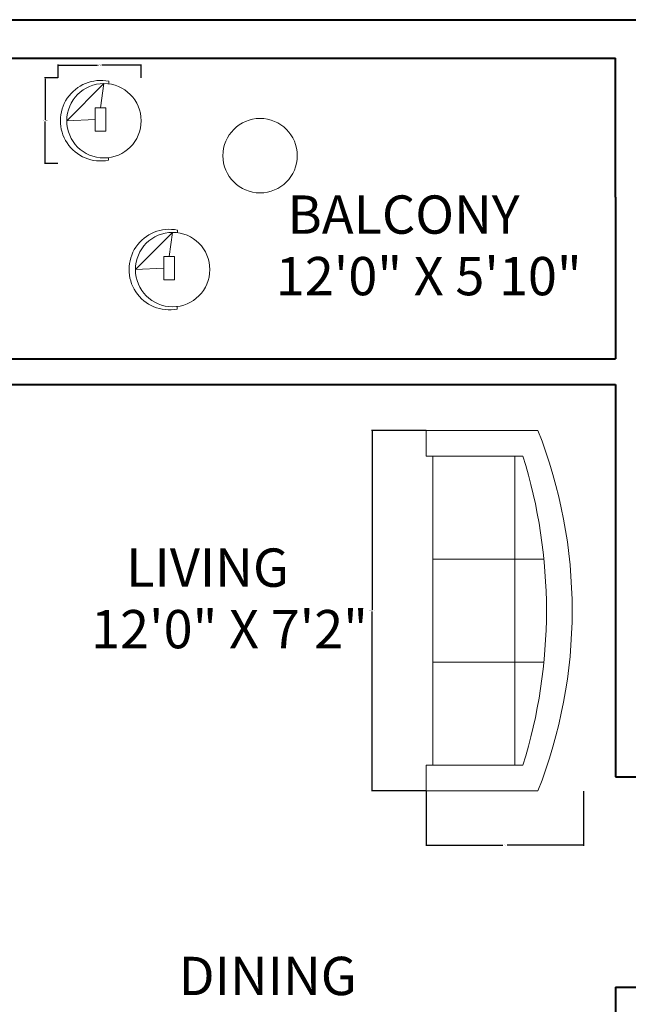
# Model space of a CAD drawing. Units: inches. Extents: x -46 to 1145, y -527 to 760.
# Tile 49 of 57: x 195 to 337, y 472 to 701. Entities that reach past the tile are written whole.
import ezdxf

# ---------------------------------------------------------------- set-up
doc = ezdxf.new("R2010")
doc.units = ezdxf.units.IN
doc.header["$MEASUREMENT"] = 0
for name, color, linetype, lineweight in [('A-ANNO-DIMS', 2, 'Continuous', 18), ('A-AREA-IDEN', 1, 'Continuous', 18), ('A-FURN', 2, 'Continuous', 13), ('WALLS', 4, 'Continuous', 40)]:
    doc.layers.add(name, color=color, linetype=linetype, lineweight=lineweight)
doc.styles.get("Standard").update_dxf_attribs({"font": 'arial.ttf'})
doc.dimstyles.get("Standard").update_dxf_attribs({"dimtxt": 0.18, "dimasz": 0.18, "dimexe": 0.18, "dimexo": 0.0625, "dimgap": 0.09, "dimtad": 0, "dimtih": 1, "dimtoh": 1, "dimdec": 0, "dimzin": 0, "dimdsep": 46, "dimlunit": 3, "dimtxsty": 'Standard', "dimcen": 0.09, "dimadec": 0, "dimazin": 0, "dimtfac": 1, "dimtdec": 0, "dimtofl": 0, "dimtmove": 0, "dimatfit": 3, "dimfxl": 1, "dimtolj": 1, "dimtzin": 0, "dimarcsym": 0})

# ---------------------------------------------------------------- blocks, each defined once
blk = doc.blocks.new('Sofa - Roundback 7 ft.')
for p, q in [((-12.00002, -32.4421), (-12.00003, -6.5971)), ((11.99997, -32.4421), (11.99998, -6.5971)), ((-36.000027, -34), (-36.000027, -11.4696)), ((-35.999844, -13.3819), (35.9998, -13.3819)), ((35.99998, -34), (35.99998, -11.4696)), ((-36.000027, -32.4421), (35.99998, -32.4421))]:
    blk.add_line(p, q)
for points in [[(-36.000027, -34), (-42.000027, -34), (-42.000027, -8)], [(41.99998, -8), (41.99998, -34), (35.99998, -34)]]:
    blk.add_lwpolyline(points)
for centre, radius, start, end in [((0, -114.25), 114.25, 68.43141, 111.5686), ((-0.00001, -127.1968), 121.1968, 72.72033, 107.2797)]:
    blk.add_arc(centre, radius, start, end)
blk = doc.blocks.new('BALCONY-CHAIR')
for p, q in [((11.28, 17.97), (11.28, 18.57)), ((1.49, 9.38), (10.16, 18.05)), ((9.33, 12.41), (10.16, 18.05)), ((8.08, 9.69), (1.49, 9.38)), ((11.2, 0.17), (11.2, 0.77))]:
    blk.add_line(p, q)
blk.add_lwpolyline([(10.57, 6.97), (8.08, 6.97), (8.08, 12.41), (10.57, 12.41)], close=True)
blk.add_circle((10.16, 9.38), 8.67)
blk.add_arc((9.38, 9.38), 9.38, 78.3491, 281.1485)
blk = doc.blocks.new('*D668')
at = {"layer": 'A-ANNO-DIMS', "color": 0, "lineweight": -2, "transparency": 16777216}
for p, q in [((289.42, 605.21), (276.7, 605.21)), ((276.88, 605.03), (276.88, 563.39)), ((276.88, 521.39), (276.88, 563.03)), ((289.42, 521.21), (276.7, 521.21))]:
    blk.add_line(p, q, dxfattribs=at)
at = {"layer": 'A-ANNO-DIMS', "color": 0, "transparency": 16777216}
for points in [[(276.85, 605.03), (276.91, 605.03), (276.88, 605.21)], [(276.85, 521.39), (276.91, 521.39), (276.88, 521.21)]]:
    blk.add_solid(points, dxfattribs=at)
at = {"layer": 'Defpoints', "color": 0, "transparency": 16777216}
for p in [(289.48, 605.21), (276.88, 521.21), (289.48, 521.21)]:
    blk.add_point(p, dxfattribs=at)
at = {"layer": 'A-ANNO-DIMS', "color": 0, "transparency": 16777216, "insert": (276.88, 563.21), "char_height": 0.18, "attachment_point": 5}
blk.add_mtext('\\A1;SOFA 84 TYP.', dxfattribs=at)
blk = doc.blocks.new('*D669')
at = {"layer": 'A-ANNO-DIMS', "color": 0, "lineweight": -2, "transparency": 16777216}
for p, q in [((289.48, 521.15), (289.48, 508.43)), ((326.15, 521.15), (326.15, 508.43)), ((289.66, 508.61), (307.29, 508.61)), ((325.97, 508.61), (308.34, 508.61))]:
    blk.add_line(p, q, dxfattribs=at)
at = {"layer": 'A-ANNO-DIMS', "color": 0, "transparency": 16777216}
for points in [[(289.66, 508.64), (289.66, 508.58), (289.48, 508.61)], [(325.97, 508.64), (325.97, 508.58), (326.15, 508.61)]]:
    blk.add_solid(points, dxfattribs=at)
at = {"layer": 'Defpoints', "color": 0, "transparency": 16777216}
for p in [(289.48, 521.21), (326.15, 521.21), (326.15, 508.61)]:
    blk.add_point(p, dxfattribs=at)
at = {"layer": 'A-ANNO-DIMS', "color": 0, "transparency": 16777216, "insert": (307.82, 508.61), "char_height": 0.18, "attachment_point": 5}
blk.add_mtext('\\A1;37 TYP.', dxfattribs=at)
blk = doc.blocks.new('*D672')
at = {"layer": 'A-ANNO-DIMS', "color": 0, "lineweight": -2, "transparency": 16777216}
for p, q in [((203.62, 687.31), (200.51, 687.31)), ((200.69, 687.13), (200.69, 677.54)), ((200.69, 667.58), (200.69, 677.17)), ((203.62, 667.4), (200.51, 667.4))]:
    blk.add_line(p, q, dxfattribs=at)
at = {"layer": 'A-ANNO-DIMS', "color": 0, "transparency": 16777216}
for points in [[(200.66, 687.13), (200.72, 687.13), (200.69, 687.31)], [(200.66, 667.58), (200.72, 667.58), (200.69, 667.4)]]:
    blk.add_solid(points, dxfattribs=at)
at = {"layer": 'Defpoints', "color": 0, "transparency": 16777216}
for p in [(200.69, 687.31), (203.68, 687.31), (203.68, 667.4)]:
    blk.add_point(p, dxfattribs=at)
at = {"layer": 'A-ANNO-DIMS', "color": 0, "transparency": 16777216, "insert": (200.69, 677.35), "char_height": 0.18, "attachment_point": 5}
blk.add_mtext('\\A1;CHAIR 20 TYP.', dxfattribs=at)
blk = doc.blocks.new('*D673')
at = {"layer": 'A-ANNO-DIMS', "color": 0, "lineweight": -2, "transparency": 16777216}
for p, q in [((203.68, 687.37), (203.68, 690.47)), ((223.04, 687.37), (223.04, 690.47)), ((203.86, 690.29), (212.84, 690.29)), ((222.86, 690.29), (213.88, 690.29))]:
    blk.add_line(p, q, dxfattribs=at)
at = {"layer": 'A-ANNO-DIMS', "color": 0, "transparency": 16777216}
for points in [[(203.86, 690.32), (203.86, 690.26), (203.68, 690.29)], [(222.86, 690.32), (222.86, 690.26), (223.04, 690.29)]]:
    blk.add_solid(points, dxfattribs=at)
at = {"layer": 'Defpoints', "color": 0, "transparency": 16777216}
for p in [(223.04, 690.29), (203.68, 687.31), (223.04, 687.31)]:
    blk.add_point(p, dxfattribs=at)
at = {"layer": 'A-ANNO-DIMS', "color": 0, "transparency": 16777216, "insert": (213.36, 690.29), "char_height": 0.18, "attachment_point": 5}
blk.add_mtext('\\A1;19 TYP.', dxfattribs=at)

msp = doc.modelspace()

# ---------------------------------------------------------------- linework, layer by layer
at = {"layer": 'A-FURN'}
msp.add_circle((250.7515, 669.2086), 8.6686, dxfattribs=at)
at = {"layer": 'WALLS'}
for p, q in [((189.5637, 700.8886), (339.5637, 700.8886)), ((189.5637, 691.8886), (333.5637, 691.8886)), ((333.5637, 659.5176), (333.5637, 691.8886)), ((333.5637, 659.5176), (333.5637, 621.8886)), ((183.5637, 621.8886), (333.5637, 621.8886)), ((183.5637, 615.8886), (333.5637, 615.8886)), ((333.5637, 615.8886), (333.5637, 524.5176)), ((333.5637, 524.5176), (394.9782, 524.5176)), ((333.5637, 475.5176), (500.0637, 475.5176)), ((333.5637, 475.5176), (333.5637, 367.232))]:
    msp.add_line(p, q, dxfattribs=at)

# ---------------------------------------------------------------- block references
at = {"layer": 'A-FURN'}
for p in [(204.215, 667.966), (220.2165, 633.2915)]:
    msp.add_blockref('BALCONY-CHAIR', p, dxfattribs=at)
at = {"layer": 'A-FURN', "rotation": 270}
msp.add_blockref('Sofa - Roundback 7 ft.', (323.483, 563.2097), dxfattribs=at)

# ---------------------------------------------------------------- texts
at = {"layer": 'A-AREA-IDEN'}
for s, height, p in [(' BALCONY', 8.92326, (254.417, 651.021)), ('12\'0" X 5\'10"', 8.923264, (254.417, 636.6866)), ('   LIVING', 8.92326, (211.3696, 568.7716)), ('12\'0" X 7\'2"', 8.923264, (211.3696, 554.4372)), ('   DINING', 8.92326, (223.6059, 473.6409))]:
    msp.add_text(s, height=height, dxfattribs=at).set_placement(p)

# ---------------------------------------------------------------- dimensions: what is measured, and where the dimension line sits
at = {"layer": 'A-ANNO-DIMS'}
for base, p1, p2, picture, middle in [((223.0427, 690.2902), (203.6777, 687.3051), (223.0427, 687.3051), '*D673', (213.3602, 690.2902)), ((326.1496, 508.6097), (289.483, 521.2097), (326.1496, 521.2097), '*D669', (307.8163, 508.6097))]:
    dim = msp.add_linear_dim(base=base, p1=p1, p2=p2, text='<> TYP.', dimstyle='Standard', override={"dimdec": 0, "dimlfac": 1, "dimrnd": 0, "dimzin": 0, "dimdsep": 46, "dimlunit": 2}, dxfattribs=at)
    dim.commit()
    dim.dimension.update_dxf_attribs({"geometry": picture, "text_midpoint": middle})
for base, p1, p2, angle, text, picture, middle in [((200.6927, 687.3051), (203.6777, 667.4046), (203.6777, 687.3051), 90, 'CHAIR <> TYP.', '*D672', (200.6927, 677.3549)), ((276.883, 521.2097), (289.483, 605.2097), (289.483, 521.2097), 270, 'SOFA <> TYP.', '*D668', (276.883, 563.2097))]:
    dim = msp.add_linear_dim(base=base, p1=p1, p2=p2, angle=angle, text=text, dimstyle='Standard', override={"dimdec": 0, "dimlfac": 1, "dimrnd": 0, "dimzin": 0, "dimdsep": 46, "dimlunit": 2}, dxfattribs=at)
    dim.commit()
    dim.dimension.update_dxf_attribs({"geometry": picture, "text_midpoint": middle})

doc.saveas('drawing.dxf')
